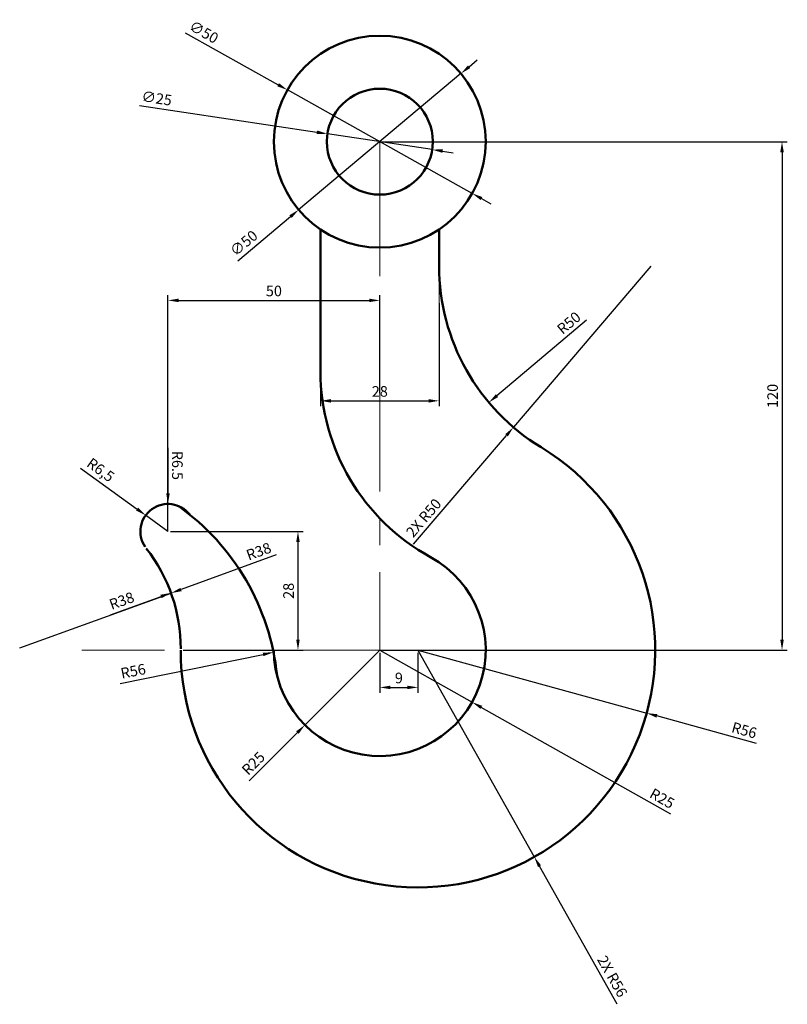
# Model space of a CAD drawing. Units: millimetres. Extents: x 3156 to 3337, y 1550 to 1782.
import ezdxf

# ---------------------------------------------------------------- set-up
doc = ezdxf.new("R2010")
doc.units = ezdxf.units.MM
doc.linetypes.add('CENTER', pattern=[50.8, 31.75, -6.35, 6.35, -6.35])
for name, color, linetype, lineweight in [('M-CNTR', 4, 'CENTER', 18), ('M-CONS', 8, 'Continuous', 13), ('M-DIMS', 2, 'Continuous', 25), ('M-OUTL', 7, 'Continuous', 50)]:
    doc.layers.add(name, color=color, linetype=linetype, lineweight=lineweight)
doc.styles.get("Standard").update_dxf_attribs({"font": 'arial.ttf'})
doc.dimstyles.new('ISO-25', dxfattribs={"dimtxt": 2.5, "dimasz": 2.5, "dimexe": 1.25, "dimexo": 0.625, "dimtad": 1, "dimtxsty": 'Standard', "dimcen": 2.5, "dimadec": 0, "dimazin": 0, "dimtfac": 1, "dimtmove": 0, "dimatfit": 3, "dimfxl": 1, "dimarcsym": 0})

# ---------------------------------------------------------------- blocks, each defined once
blk = doc.blocks.new('*D1')
at = {"layer": 'Defpoints', "color": 0, "transparency": 16777216}
for p in [(3240.63, 1753.47), (3240.63, 1633.47), (3335.56, 1633.47)]:
    blk.add_point(p, dxfattribs=at)
at = {"layer": 'M-DIMS', "color": 0, "lineweight": -2, "transparency": 16777216}
for p, q in [((3241.25, 1753.47), (3336.81, 1753.47)), ((3335.56, 1750.97), (3335.56, 1635.97)), ((3241.25, 1633.47), (3336.81, 1633.47))]:
    blk.add_line(p, q, dxfattribs=at)
at = {"layer": 'M-DIMS', "color": 0, "transparency": 16777216}
for points in [[(3335.14, 1750.97), (3335.98, 1750.97), (3335.56, 1753.47)], [(3335.14, 1635.97), (3335.98, 1635.97), (3335.56, 1633.47)]]:
    blk.add_solid(points, dxfattribs=at)
at = {"layer": 'M-DIMS', "color": 0, "transparency": 16777216, "insert": (3333.66, 1693.47), "char_height": 2.5, "attachment_point": 5, "rotation": 90}
blk.add_mtext('120', dxfattribs=at)
blk = doc.blocks.new('*D2')
at = {"layer": 'Defpoints', "color": 0, "transparency": 16777216}
for p in [(3240.63, 1633.47), (3249.63, 1633.47), (3249.63, 1624.68)]:
    blk.add_point(p, dxfattribs=at)
at = {"layer": 'M-DIMS', "color": 0, "lineweight": -2, "transparency": 16777216}
for p, q in [((3240.63, 1632.85), (3240.63, 1623.43)), ((3249.63, 1632.85), (3249.63, 1623.43)), ((3243.13, 1624.68), (3247.13, 1624.68))]:
    blk.add_line(p, q, dxfattribs=at)
at = {"layer": 'M-DIMS', "color": 0, "transparency": 16777216}
for points in [[(3243.13, 1625.09), (3243.13, 1624.26), (3240.63, 1624.68)], [(3247.13, 1625.09), (3247.13, 1624.26), (3249.63, 1624.68)]]:
    blk.add_solid(points, dxfattribs=at)
at = {"layer": 'M-DIMS', "color": 0, "transparency": 16777216, "insert": (3245.13, 1626.58), "char_height": 2.5, "attachment_point": 5}
blk.add_mtext('9', dxfattribs=at)
blk = doc.blocks.new('*D3')
at = {"layer": 'Defpoints', "color": 0, "transparency": 16777216}
for p in [(3190.63, 1661.47), (3193.63, 1633.47), (3221.31, 1633.47)]:
    blk.add_point(p, dxfattribs=at)
at = {"layer": 'M-DIMS', "color": 0, "lineweight": -2, "transparency": 16777216}
for p, q in [((3191.25, 1661.47), (3222.56, 1661.47)), ((3221.31, 1658.97), (3221.31, 1635.97)), ((3194.25, 1633.47), (3222.56, 1633.47))]:
    blk.add_line(p, q, dxfattribs=at)
at = {"layer": 'M-DIMS', "color": 0, "transparency": 16777216}
for points in [[(3220.89, 1658.97), (3221.72, 1658.97), (3221.31, 1661.47)], [(3220.89, 1635.97), (3221.72, 1635.97), (3221.31, 1633.47)]]:
    blk.add_solid(points, dxfattribs=at)
at = {"layer": 'M-DIMS', "color": 0, "transparency": 16777216, "insert": (3219.41, 1647.47), "char_height": 2.5, "attachment_point": 5, "rotation": 90}
blk.add_mtext('28', dxfattribs=at)
blk = doc.blocks.new('*D4')
at = {"layer": 'Defpoints', "color": 0, "transparency": 16777216}
for p in [(3240.63, 1716.01), (3240.63, 1693.47), (3190.63, 1661.47)]:
    blk.add_point(p, dxfattribs=at)
at = {"layer": 'M-DIMS', "color": 0, "lineweight": -2, "transparency": 16777216}
for p, q in [((3190.63, 1662.1), (3190.63, 1717.26)), ((3240.63, 1694.1), (3240.63, 1717.26)), ((3193.13, 1716.01), (3238.13, 1716.01))]:
    blk.add_line(p, q, dxfattribs=at)
at = {"layer": 'M-DIMS', "color": 0, "transparency": 16777216}
for points in [[(3193.13, 1716.43), (3193.13, 1715.6), (3190.63, 1716.01)], [(3238.13, 1716.43), (3238.13, 1715.6), (3240.63, 1716.01)]]:
    blk.add_solid(points, dxfattribs=at)
at = {"layer": 'M-DIMS', "color": 0, "transparency": 16777216, "insert": (3215.63, 1717.92), "char_height": 2.5, "attachment_point": 5}
blk.add_mtext('50', dxfattribs=at)
blk = doc.blocks.new('*D5')
at = {"layer": 'Defpoints', "color": 0, "transparency": 16777216}
for p in [(3191.34, 1646.99), (3155.63, 1633.99)]:
    blk.add_point(p, dxfattribs=at)
at = {"layer": 'M-DIMS', "color": 0, "lineweight": -2, "transparency": 16777216}
blk.add_line((3177.07, 1641.79), (3188.99, 1646.13), dxfattribs=at)
at = {"layer": 'M-DIMS', "color": 0, "transparency": 16777216}
blk.add_solid([(3188.84, 1646.53), (3189.13, 1645.74), (3191.34, 1646.99)], dxfattribs=at)
at = {"layer": 'M-DIMS', "color": 0, "transparency": 16777216, "insert": (3179.81, 1644.82), "char_height": 2.5, "attachment_point": 5, "rotation": 20.0032}
blk.add_mtext('R38', dxfattribs=at)
blk = doc.blocks.new('*D6')
at = {"layer": 'Defpoints', "color": 0, "transparency": 16777216}
for p in [(3215.53, 1632.96), (3160.64, 1621.84)]:
    blk.add_point(p, dxfattribs=at)
at = {"layer": 'M-DIMS', "color": 0, "lineweight": -2, "transparency": 16777216}
blk.add_line((3179.31, 1625.62), (3213.08, 1632.46), dxfattribs=at)
at = {"layer": 'M-DIMS', "color": 0, "transparency": 16777216}
blk.add_solid([(3213, 1632.87), (3213.16, 1632.05), (3215.53, 1632.96)], dxfattribs=at)
at = {"layer": 'M-DIMS', "color": 0, "transparency": 16777216, "insert": (3182.47, 1628.2), "char_height": 2.5, "attachment_point": 5, "rotation": 11.4435}
blk.add_mtext('R56', dxfattribs=at)
blk = doc.blocks.new('*D7')
at = {"layer": 'Defpoints', "color": 0, "transparency": 16777216}
for p in [(3185.36, 1665.29), (3190.63, 1661.47)]:
    blk.add_point(p, dxfattribs=at)
at = {"layer": 'M-DIMS', "color": 0, "lineweight": -2, "transparency": 16777216}
for p, q in [((3169.98, 1676.44), (3183.34, 1666.75)), ((3190.63, 1661.47), (3185.36, 1665.29))]:
    blk.add_line(p, q, dxfattribs=at)
at = {"layer": 'M-DIMS', "color": 0, "transparency": 16777216}
blk.add_solid([(3183.58, 1667.09), (3183.09, 1666.42), (3185.36, 1665.29)], dxfattribs=at)
at = {"layer": 'M-DIMS', "color": 0, "transparency": 16777216, "insert": (3174.55, 1675.75), "char_height": 2.5, "attachment_point": 5, "rotation": 324.0691}
blk.add_mtext('R6,5', dxfattribs=at)
blk = doc.blocks.new('*D8')
at = {"layer": 'Defpoints', "color": 0, "transparency": 16777216}
for p in [(3240.63, 1633.47), (3262.41, 1621.2)]:
    blk.add_point(p, dxfattribs=at)
at = {"layer": 'M-DIMS', "color": 0, "lineweight": -2, "transparency": 16777216}
for p, q in [((3240.63, 1633.47), (3262.41, 1621.2)), ((3309.32, 1594.76), (3264.58, 1619.97))]:
    blk.add_line(p, q, dxfattribs=at)
at = {"layer": 'M-DIMS', "color": 0, "transparency": 16777216}
blk.add_solid([(3264.79, 1620.33), (3264.38, 1619.61), (3262.41, 1621.2)], dxfattribs=at)
at = {"layer": 'M-DIMS', "color": 0, "transparency": 16777216, "insert": (3307.1, 1598.19), "char_height": 2.5, "attachment_point": 5, "rotation": 330.5957}
blk.add_mtext('R25', dxfattribs=at)
blk = doc.blocks.new('*D9')
at = {"layer": 'Defpoints', "color": 0, "transparency": 16777216}
for p in [(3249.63, 1633.47), (3303.62, 1618.61)]:
    blk.add_point(p, dxfattribs=at)
at = {"layer": 'M-DIMS', "color": 0, "lineweight": -2, "transparency": 16777216}
for p, q in [((3249.63, 1633.47), (3303.62, 1618.61)), ((3329.54, 1611.47), (3306.03, 1617.95))]:
    blk.add_line(p, q, dxfattribs=at)
at = {"layer": 'M-DIMS', "color": 0, "transparency": 16777216}
blk.add_solid([(3306.14, 1618.35), (3305.92, 1617.54), (3303.62, 1618.61)], dxfattribs=at)
at = {"layer": 'M-DIMS', "color": 0, "transparency": 16777216, "insert": (3326.56, 1614.26), "char_height": 2.5, "attachment_point": 5, "rotation": 344.6077}
blk.add_mtext('R56', dxfattribs=at)
blk = doc.blocks.new('*D10')
at = {"layer": 'Defpoints', "color": 0, "transparency": 16777216}
for p in [(3304.63, 1724.09), (3266.35, 1691.91)]:
    blk.add_point(p, dxfattribs=at)
at = {"layer": 'M-DIMS', "color": 0, "lineweight": -2, "transparency": 16777216}
blk.add_line((3289.44, 1711.32), (3268.27, 1693.52), dxfattribs=at)
at = {"layer": 'M-DIMS', "color": 0, "transparency": 16777216}
blk.add_solid([(3268, 1693.84), (3268.54, 1693.2), (3266.35, 1691.91)], dxfattribs=at)
at = {"layer": 'M-DIMS', "color": 0, "transparency": 16777216, "insert": (3285.45, 1710.45), "char_height": 2.5, "attachment_point": 5, "rotation": 40.0525}
blk.add_mtext('R50', dxfattribs=at)
blk = doc.blocks.new('*D11')
at = {"layer": 'Defpoints', "color": 0, "transparency": 16777216}
for p in [(3226.63, 1716.01), (3254.63, 1716.01), (3254.63, 1692.31)]:
    blk.add_point(p, dxfattribs=at)
at = {"layer": 'M-DIMS', "color": 0, "lineweight": -2, "transparency": 16777216}
for p, q in [((3226.63, 1715.39), (3226.63, 1691.06)), ((3254.63, 1715.39), (3254.63, 1691.06)), ((3229.13, 1692.31), (3252.13, 1692.31))]:
    blk.add_line(p, q, dxfattribs=at)
at = {"layer": 'M-DIMS', "color": 0, "transparency": 16777216}
for points in [[(3229.13, 1692.72), (3229.13, 1691.89), (3226.63, 1692.31)], [(3252.13, 1692.72), (3252.13, 1691.89), (3254.63, 1692.31)]]:
    blk.add_solid(points, dxfattribs=at)
at = {"layer": 'M-DIMS', "color": 0, "transparency": 16777216, "insert": (3240.63, 1694.21), "char_height": 2.5, "attachment_point": 5}
blk.add_mtext('28', dxfattribs=at)
blk = doc.blocks.new('*D12')
at = {"layer": 'Defpoints', "color": 0, "transparency": 16777216}
for p in [(3228.27, 1755.33), (3252.99, 1751.61)]:
    blk.add_point(p, dxfattribs=at)
at = {"layer": 'M-DIMS', "color": 0, "lineweight": -2, "transparency": 16777216}
for p, q in [((3183.88, 1762.02), (3225.79, 1755.71)), ((3252.99, 1751.61), (3228.27, 1755.33)), ((3255.46, 1751.24), (3257.93, 1750.87))]:
    blk.add_line(p, q, dxfattribs=at)
at = {"layer": 'M-DIMS', "color": 0, "transparency": 16777216}
for points in [[(3225.86, 1756.12), (3225.73, 1755.3), (3228.27, 1755.33)], [(3255.52, 1751.65), (3255.4, 1750.83), (3252.99, 1751.61)]]:
    blk.add_solid(points, dxfattribs=at)
at = {"layer": 'M-DIMS', "color": 0, "transparency": 16777216, "insert": (3187.92, 1763.4), "char_height": 2.5, "attachment_point": 5, "rotation": 351.4361}
blk.add_mtext('∅25', dxfattribs=at)
blk = doc.blocks.new('*D13')
at = {"layer": 'Defpoints', "color": 0, "transparency": 16777216}
for p in [(3218.81, 1765.68), (3262.44, 1741.26)]:
    blk.add_point(p, dxfattribs=at)
at = {"layer": 'M-DIMS', "color": 0, "lineweight": -2, "transparency": 16777216}
for p, q in [((3194.68, 1779.19), (3216.63, 1766.91)), ((3262.44, 1741.26), (3218.81, 1765.68)), ((3264.62, 1740.04), (3266.8, 1738.82))]:
    blk.add_line(p, q, dxfattribs=at)
at = {"layer": 'M-DIMS', "color": 0, "transparency": 16777216}
for points in [[(3216.83, 1767.27), (3216.43, 1766.54), (3218.81, 1765.68)], [(3264.83, 1740.41), (3264.42, 1739.68), (3262.44, 1741.26)]]:
    blk.add_solid(points, dxfattribs=at)
at = {"layer": 'M-DIMS', "color": 0, "transparency": 16777216, "insert": (3198.93, 1779.07), "char_height": 2.5, "attachment_point": 5, "rotation": 330.7632}
blk.add_mtext('∅50', dxfattribs=at)
blk = doc.blocks.new('*D14')
at = {"layer": 'Defpoints', "color": 0, "transparency": 16777216}
for p in [(3259.78, 1769.54), (3221.47, 1737.4)]:
    blk.add_point(p, dxfattribs=at)
at = {"layer": 'M-DIMS', "color": 0, "lineweight": -2, "transparency": 16777216}
for p, q in [((3261.69, 1771.15), (3263.61, 1772.76)), ((3259.78, 1769.54), (3221.47, 1737.4)), ((3207.09, 1725.34), (3219.56, 1735.8))]:
    blk.add_line(p, q, dxfattribs=at)
at = {"layer": 'M-DIMS', "color": 0, "transparency": 16777216}
for points in [[(3261.43, 1771.47), (3261.96, 1770.83), (3259.78, 1769.54)], [(3219.29, 1736.12), (3219.83, 1735.48), (3221.47, 1737.4)]]:
    blk.add_solid(points, dxfattribs=at)
at = {"layer": 'M-DIMS', "color": 0, "transparency": 16777216, "insert": (3208.72, 1729.27), "char_height": 2.5, "attachment_point": 5, "rotation": 39.9978}
blk.add_mtext('∅50', dxfattribs=at)
blk = doc.blocks.new('*D15')
at = {"layer": 'Defpoints', "color": 0, "transparency": 16777216}
for p in [(3304.63, 1724.09), (3272.16, 1686.06)]:
    blk.add_point(p, dxfattribs=at)
at = {"layer": 'M-DIMS', "color": 0, "lineweight": -2, "transparency": 16777216}
for p, q in [((3304.63, 1724.09), (3272.16, 1686.06)), ((3248.58, 1658.45), (3270.54, 1684.16))]:
    blk.add_line(p, q, dxfattribs=at)
at = {"layer": 'M-DIMS', "color": 0, "transparency": 16777216}
blk.add_solid([(3270.22, 1684.43), (3270.85, 1683.89), (3272.16, 1686.06)], dxfattribs=at)
at = {"layer": 'M-DIMS', "color": 0, "transparency": 16777216, "insert": (3251.23, 1664.48), "char_height": 2.5, "attachment_point": 5, "rotation": 49.5086}
blk.add_mtext('2X R50', dxfattribs=at)
blk = doc.blocks.new('*D16')
at = {"layer": 'Defpoints', "color": 0, "transparency": 16777216}
for p in [(3190.63, 1667.97), (3190.63, 1661.47)]:
    blk.add_point(p, dxfattribs=at)
at = {"layer": 'M-DIMS', "color": 0, "lineweight": -2, "transparency": 16777216}
for p, q in [((3190.63, 1681.19), (3190.63, 1670.47)), ((3190.63, 1661.47), (3190.63, 1667.97))]:
    blk.add_line(p, q, dxfattribs=at)
at = {"layer": 'M-DIMS', "color": 0, "transparency": 16777216}
blk.add_solid([(3191.04, 1670.47), (3190.21, 1670.47), (3190.63, 1667.97)], dxfattribs=at)
at = {"layer": 'M-DIMS', "color": 0, "transparency": 16777216, "insert": (3192.53, 1677.08), "char_height": 2.5, "attachment_point": 5, "rotation": 270.0025}
blk.add_mtext('R6.5', dxfattribs=at)
blk = doc.blocks.new('*D17')
at = {"layer": 'Defpoints', "color": 0, "transparency": 16777216}
for p in [(3240.63, 1633.47), (3222.95, 1615.8)]:
    blk.add_point(p, dxfattribs=at)
at = {"layer": 'M-DIMS', "color": 0, "lineweight": -2, "transparency": 16777216}
for p, q in [((3240.63, 1633.47), (3222.95, 1615.8)), ((3209.78, 1602.63), (3221.18, 1614.03))]:
    blk.add_line(p, q, dxfattribs=at)
at = {"layer": 'M-DIMS', "color": 0, "transparency": 16777216}
blk.add_solid([(3220.89, 1614.32), (3221.48, 1613.73), (3222.95, 1615.8)], dxfattribs=at)
at = {"layer": 'M-DIMS', "color": 0, "transparency": 16777216, "insert": (3211, 1606.53), "char_height": 2.5, "attachment_point": 5, "rotation": 44.9988}
blk.add_mtext('R25', dxfattribs=at)
blk = doc.blocks.new('*D18')
at = {"layer": 'Defpoints', "color": 0, "transparency": 16777216}
for p in [(3249.63, 1633.47), (3277.09, 1584.67)]:
    blk.add_point(p, dxfattribs=at)
at = {"layer": 'M-DIMS', "color": 0, "lineweight": -2, "transparency": 16777216}
for p, q in [((3249.63, 1633.47), (3277.09, 1584.67)), ((3296.67, 1549.89), (3278.32, 1582.49))]:
    blk.add_line(p, q, dxfattribs=at)
at = {"layer": 'M-DIMS', "color": 0, "transparency": 16777216}
blk.add_solid([(3278.68, 1582.7), (3277.96, 1582.29), (3277.09, 1584.67)], dxfattribs=at)
at = {"layer": 'M-DIMS', "color": 0, "transparency": 16777216, "insert": (3295.23, 1556.32), "char_height": 2.5, "attachment_point": 5, "rotation": 299.3719}
blk.add_mtext('2X R56', dxfattribs=at)
blk = doc.blocks.new('*D19')
at = {"layer": 'Defpoints', "color": 0, "transparency": 16777216}
for p in [(3191.36, 1646.93), (3155.63, 1633.99)]:
    blk.add_point(p, dxfattribs=at)
at = {"layer": 'M-DIMS', "color": 0, "lineweight": -2, "transparency": 16777216}
for p, q in [((3216.19, 1655.93), (3193.71, 1647.78)), ((3155.63, 1633.99), (3191.36, 1646.93))]:
    blk.add_line(p, q, dxfattribs=at)
at = {"layer": 'M-DIMS', "color": 0, "transparency": 16777216}
blk.add_solid([(3193.56, 1648.17), (3193.85, 1647.39), (3191.36, 1646.93)], dxfattribs=at)
at = {"layer": 'M-DIMS', "color": 0, "transparency": 16777216, "insert": (3212.15, 1656.48), "char_height": 2.5, "attachment_point": 5, "rotation": 19.911}
blk.add_mtext('R38', dxfattribs=at)

msp = doc.modelspace()

# ---------------------------------------------------------------- linework, layer by layer
at = {"layer": 'M-CNTR'}
for p, q in [((3240.626, 1753.474), (3240.626, 1633.474)), ((3240.626, 1633.474), (3170.283, 1633.474)), ((3240.626, 1633.474), (3315.658, 1633.474))]:
    msp.add_line(p, q, dxfattribs=at)
at = {"layer": 'M-CONS'}
for p, q in [((3226.626, 1732.761), (3226.626, 1704.761)), ((3254.626, 1704.761), (3254.626, 1732.761)), ((3254.626, 1654.192), (3254.626, 1654.186)), ((3240.626, 1633.474), (3249.626, 1633.474))]:
    msp.add_line(p, q, dxfattribs=at)
at = {"layer": 'M-OUTL'}
for p, q in [((3226.626, 1732.761), (3226.626, 1699.269)), ((3254.626, 1724.088), (3254.626, 1732.761))]:
    msp.add_line(p, q, dxfattribs=at)
for radius in [25, 12.5]:
    msp.add_circle((3240.626, 1753.474), radius, dxfattribs=at)
for centre, radius, start, end in [((3304.626, 1724.088), 50, 180, 238.74366), ((3276.626, 1699.269), 50, 180, 241.3146), ((3249.626, 1633.474), 56, 180, 58.74366), ((3190.626, 1661.474), 6.5, 38.00609, 213.81179), ((3160.643, 1621.845), 56, 5.74993, 54.59712), ((3155.628, 1633.99), 38, 359.68525, 38.14177), ((3240.626, 1633.474), 25, 180, 61.3146)]:
    msp.add_arc(centre, radius, start, end, dxfattribs=at)

# ---------------------------------------------------------------- dimensions: what is measured, and where the dimension line sits
at = {"layer": 'M-DIMS'}
for p1, p2, override, picture, middle in [((3262.441, 1741.263), (3218.811, 1765.684), {"dimclrd": 0, "dimclre": 0, "dimclrt": 0}, '*D13', (3197.967, 1777.351)), ((3259.778, 1769.543), (3221.475, 1737.405), {"dimdec": 0, "dimlfac": 1, "dimrnd": 0, "dimzin": 0, "dimdsep": 46, "dimlunit": 2}, '*D14', (3209.984, 1727.763)), ((3252.987, 1751.612), (3228.266, 1755.335), {"dimclrd": 0, "dimclre": 0, "dimclrt": 0}, '*D12', (3187.624, 1761.455))]:
    dim = msp.add_diameter_dim_2p(p1=p1, p2=p2, dimstyle='ISO-25', override=override, dxfattribs=at)
    dim.commit()
    dim.dimension.update_dxf_attribs({"geometry": picture, "text_midpoint": middle, "dimtype": 163})
for base, p1, p2, picture, middle in [((3335.559, 1633.474), (3240.626, 1753.474), (3240.626, 1633.474), '*D1', (3333.657, 1693.474)), ((3221.307, 1633.474), (3190.626, 1661.474), (3193.626, 1633.474), '*D3', (3219.406, 1647.474))]:
    dim = msp.add_linear_dim(base=base, p1=p1, p2=p2, angle=90, dimstyle='ISO-25', override={"dimclrd": 0, "dimclre": 0, "dimclrt": 0}, dxfattribs=at)
    dim.commit()
    dim.dimension.update_dxf_attribs({"geometry": picture, "text_midpoint": middle})
for center, mpoint, picture, middle in [((3304.626, 1724.088), (3272.16, 1686.063), '*D15', (3252.68, 1663.248)), ((3249.626, 1633.474), (3277.093, 1584.672), '*D18', (3293.573, 1555.391))]:
    dim = msp.add_radius_dim(center=center, mpoint=mpoint, text='2X <>', dimstyle='ISO-25', override={"dimdec": 0, "dimlfac": 1, "dimrnd": 0, "dimzin": 0, "dimdsep": 46, "dimlunit": 2}, dxfattribs=at)
    dim.commit()
    dim.dimension.update_dxf_attribs({"geometry": picture, "text_midpoint": middle, "dimtype": 164})
for center, mpoint, override, picture, middle in [((3304.626, 1724.088), (3266.354, 1691.914), {"dimclrd": 0, "dimclre": 0, "dimclrt": 0}, '*D10', (3286.677, 1708.999)), ((3190.626, 1661.474), (3185.363, 1665.288), {"dimclrd": 0, "dimclre": 0, "dimclrt": 0}, '*D7', (3173.303, 1674.028)), ((3155.628, 1633.99), (3191.356, 1646.931), {"dimdec": 0, "dimlfac": 1, "dimrnd": 0, "dimzin": 0, "dimdsep": 46, "dimlunit": 2}, '*D19', (3212.793, 1654.696)), ((3155.628, 1633.99), (3191.335, 1646.989), {"dimclrd": 0, "dimclre": 0, "dimclrt": 0}, '*D5', (3180.463, 1643.031)), ((3160.643, 1621.845), (3215.53, 1632.956), {"dimclrd": 0, "dimclre": 0, "dimclrt": 0}, '*D6', (3182.85, 1626.34)), ((3240.626, 1633.474), (3222.948, 1615.796), {"dimdec": 0, "dimlfac": 1, "dimrnd": 0, "dimzin": 0, "dimdsep": 46, "dimlunit": 2}, '*D17', (3212.341, 1605.19)), ((3240.626, 1633.474), (3262.406, 1621.199), {"dimclrd": 0, "dimclre": 0, "dimclrt": 0}, '*D8', (3306.169, 1596.535)), ((3249.626, 1633.474), (3303.618, 1618.61), {"dimclrd": 0, "dimclre": 0, "dimclrt": 0}, '*D9', (3326.06, 1612.431))]:
    dim = msp.add_radius_dim(center=center, mpoint=mpoint, dimstyle='ISO-25', override=override, dxfattribs=at)
    dim.commit()
    dim.dimension.update_dxf_attribs({"geometry": picture, "text_midpoint": middle, "dimtype": 164})
for base, p1, p2, picture, middle in [((3240.626, 1716.015), (3190.626, 1661.474), (3240.626, 1693.474), '*D4', (3215.626, 1717.916)), ((3254.626, 1692.308), (3226.626, 1716.015), (3254.626, 1716.015), '*D11', (3240.626, 1694.21)), ((3249.626, 1624.678), (3240.626, 1633.474), (3249.626, 1633.474), '*D2', (3245.126, 1626.58))]:
    dim = msp.add_linear_dim(base=base, p1=p1, p2=p2, dimstyle='ISO-25', override={"dimclrd": 0, "dimclre": 0, "dimclrt": 0}, dxfattribs=at)
    dim.commit()
    dim.dimension.update_dxf_attribs({"geometry": picture, "text_midpoint": middle})
dim = msp.add_radius_dim(center=(3190.626, 1661.474), mpoint=(3190.626, 1667.974), dimstyle='ISO-25', override={"dimdec": 1, "dimlfac": 1, "dimrnd": 0, "dimzin": 0, "dimdsep": 46, "dimlunit": 2}, dxfattribs=at)
dim.commit()
dim.dimension.update_dxf_attribs({"geometry": '*D16', "text_midpoint": (3192.527, 1677.08)})

doc.saveas('drawing.dxf')
